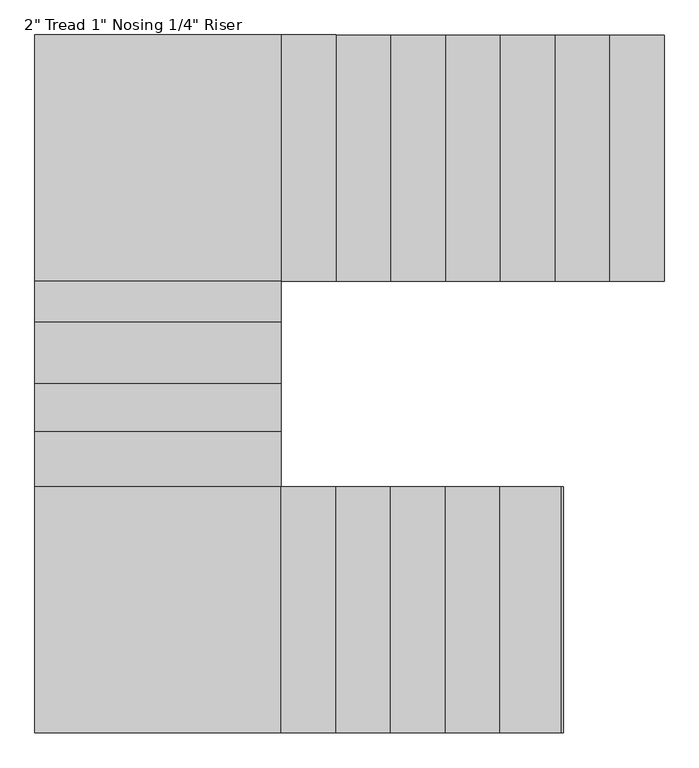
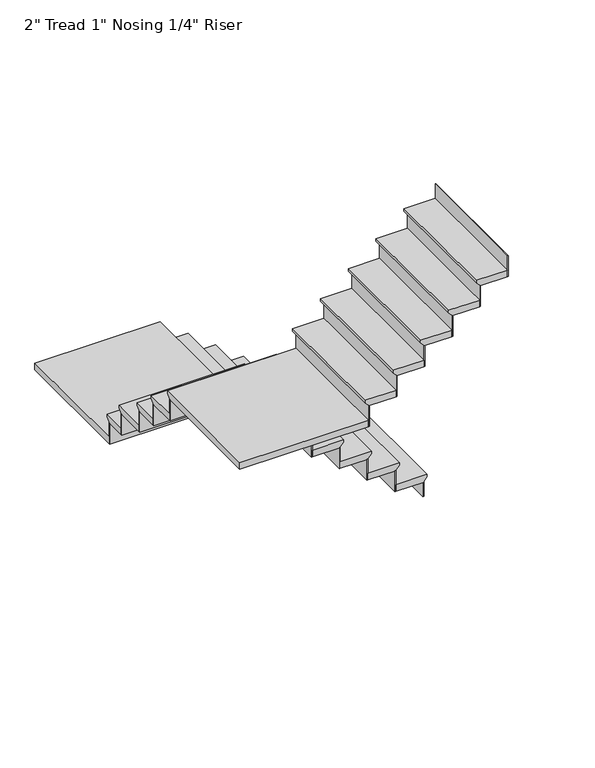
"""IFC4 building model written with IfcOpenShell, lengths in millimetres: stair flight geometry."""

from ifc_helpers import new_model, si_unit, origin, place, context, project, spatial, faceted_brep, source, transform, mapped, element, save


def stair_flight_dc8f8b64(model_context):
    return source(origin(), model_context, "Body", "Brep", [
        faceted_brep([(-3603.1340247, 922.0319954, 16143.3710526), (-3603.1340247, 922.0319954, 16162.4210526), (-3603.1340247, 7.6319954, 16162.4210526), (-3603.1340247, 7.6319954, 16143.3710526), (-3628.5340247, 922.0319954, 16117.9710526), (-3628.5340247, 7.6319954, 16117.9710526), (-3831.7340247, 922.0319954, 16162.4210526), (-3831.7340247, 7.6319954, 16162.4210526), (-3628.5340247, 7.6319954, 16111.6210526), (-3831.7340247, 7.6319954, 16111.6210526), (-3831.7340247, 922.0319954, 16111.6210526), (-3628.5340247, 922.0319954, 16111.6210526)], [[[0, 1, 2, 3]], [[4, 0, 3, 5]], [[2, 1, 6, 7]], [[8, 9, 10, 11]], [[2, 7, 9, 8, 5, 3]], [[8, 11, 4, 5]], [[6, 1, 0, 4, 11, 10]], [[7, 6, 10, 9]]]),
        faceted_brep([(-3628.5340247, 922.0319954, 16111.6210526), (-3628.5340247, 922.0319954, 16002.0), (-3634.8840247, 922.0319954, 16002.0), (-3634.8840247, 922.0319954, 16111.6210526), (-3628.5340247, 7.6319954, 16111.6210526), (-3634.8840247, 7.6319954, 16111.6210526), (-3634.8840247, 7.6319954, 16002.0), (-3628.5340247, 7.6319954, 16002.0)], [[[0, 1, 2, 3]], [[4, 5, 6, 7]], [[1, 0, 4, 7]], [[2, 1, 7, 6]], [[3, 2, 6, 5]], [[0, 3, 5, 4]]]),
        faceted_brep([(-3831.7340247, 922.0319954, 16272.0421053), (-3831.7340247, 922.0319954, 16111.6210526), (-3838.0840247, 922.0319954, 16111.6210526), (-3838.0840247, 922.0319954, 16272.0421053), (-3831.7340247, 7.6319954, 16272.0421053), (-3838.0840247, 7.6319954, 16272.0421053), (-3838.0840247, 7.6319954, 16111.6210526), (-3831.7340247, 7.6319954, 16111.6210526)], [[[0, 1, 2, 3]], [[4, 5, 6, 7]], [[1, 0, 4, 7]], [[2, 1, 7, 6]], [[3, 2, 6, 5]], [[0, 3, 5, 4]]]),
        faceted_brep([(-3806.3340247, 7.6319954, 16322.8421053), (-3806.3340247, 922.0319954, 16322.8421053), (-4034.9340247, 922.0319954, 16322.8421053), (-4034.9340247, 7.6319954, 16322.8421053), (-3831.7340247, 7.6319954, 16272.0421053), (-4034.9340247, 7.6319954, 16272.0421053), (-4034.9340247, 922.0319954, 16272.0421053), (-3831.7340247, 922.0319954, 16272.0421053), (-3831.7340247, 7.6319954, 16278.3921053), (-3806.3340247, 7.6319954, 16303.7921053), (-3831.7340247, 922.0319954, 16278.3921053), (-3806.3340247, 922.0319954, 16303.7921053)], [[[0, 1, 2, 3]], [[4, 5, 6, 7]], [[0, 3, 5, 4, 8, 9]], [[4, 7, 10, 8]], [[2, 1, 11, 10, 7, 6]], [[3, 2, 6, 5]], [[11, 1, 0, 9]], [[10, 11, 9, 8]]]),
        faceted_brep([(-4034.9340247, 922.0319954, 16432.4631579), (-4034.9340247, 922.0319954, 16272.0421053), (-4041.2840247, 922.0319954, 16272.0421053), (-4041.2840247, 922.0319954, 16432.4631579), (-4034.9340247, 7.6319954, 16432.4631579), (-4041.2840247, 7.6319954, 16432.4631579), (-4041.2840247, 7.6319954, 16272.0421053), (-4034.9340247, 7.6319954, 16272.0421053)], [[[0, 1, 2, 3]], [[4, 5, 6, 7]], [[1, 0, 4, 7]], [[2, 1, 7, 6]], [[3, 2, 6, 5]], [[0, 3, 5, 4]]]),
        faceted_brep([(-4009.5340247, 7.6319954, 16483.2631579), (-4009.5340247, 922.0319954, 16483.2631579), (-4238.1340247, 922.0319954, 16483.2631579), (-4238.1340247, 7.6319954, 16483.2631579), (-4034.9340247, 7.6319954, 16432.4631579), (-4238.1340247, 7.6319954, 16432.4631579), (-4238.1340247, 922.0319954, 16432.4631579), (-4034.9340247, 922.0319954, 16432.4631579), (-4034.9340247, 7.6319954, 16438.8131579), (-4009.5340247, 7.6319954, 16464.2131579), (-4034.9340247, 922.0319954, 16438.8131579), (-4009.5340247, 922.0319954, 16464.2131579)], [[[0, 1, 2, 3]], [[4, 5, 6, 7]], [[0, 3, 5, 4, 8, 9]], [[4, 7, 10, 8]], [[2, 1, 11, 10, 7, 6]], [[3, 2, 6, 5]], [[11, 1, 0, 9]], [[10, 11, 9, 8]]]),
        faceted_brep([(-4238.1340247, 922.0319954, 16592.8842105), (-4238.1340247, 922.0319954, 16432.4631579), (-4244.4840247, 922.0319954, 16432.4631579), (-4244.4840247, 922.0319954, 16592.8842105), (-4238.1340247, 7.6319954, 16592.8842105), (-4244.4840247, 7.6319954, 16592.8842105), (-4244.4840247, 7.6319954, 16432.4631579), (-4238.1340247, 7.6319954, 16432.4631579)], [[[0, 1, 2, 3]], [[4, 5, 6, 7]], [[1, 0, 4, 7]], [[2, 1, 7, 6]], [[3, 2, 6, 5]], [[0, 3, 5, 4]]]),
        faceted_brep([(-4212.7340247, 7.6319954, 16643.6842105), (-4212.7340247, 922.0319954, 16643.6842105), (-4441.3340247, 922.0319954, 16643.6842105), (-4441.3340247, 7.6319954, 16643.6842105), (-4238.1340247, 7.6319954, 16592.8842105), (-4441.3340247, 7.6319954, 16592.8842105), (-4441.3340247, 922.0319954, 16592.8842105), (-4238.1340247, 922.0319954, 16592.8842105), (-4238.1340247, 7.6319954, 16599.2342105), (-4212.7340247, 7.6319954, 16624.6342105), (-4238.1340247, 922.0319954, 16599.2342105), (-4212.7340247, 922.0319954, 16624.6342105)], [[[0, 1, 2, 3]], [[4, 5, 6, 7]], [[0, 3, 5, 4, 8, 9]], [[4, 7, 10, 8]], [[2, 1, 11, 10, 7, 6]], [[3, 2, 6, 5]], [[11, 1, 0, 9]], [[10, 11, 9, 8]]]),
        faceted_brep([(-4441.3340247, 922.0319954, 16753.3052632), (-4441.3340247, 922.0319954, 16592.8842105), (-4447.6840247, 922.0319954, 16592.8842105), (-4447.6840247, 922.0319954, 16753.3052632), (-4441.3340247, 7.6319954, 16753.3052632), (-4447.6840247, 7.6319954, 16753.3052632), (-4447.6840247, 7.6319954, 16592.8842105), (-4441.3340247, 7.6319954, 16592.8842105)], [[[0, 1, 2, 3]], [[4, 5, 6, 7]], [[1, 0, 4, 7]], [[2, 1, 7, 6]], [[3, 2, 6, 5]], [[0, 3, 5, 4]]]),
        faceted_brep([(-4415.9340247, 7.6319954, 16804.1052632), (-4415.9340247, 922.0319954, 16804.1052632), (-4644.5340247, 922.0319954, 16804.1052632), (-4644.5340247, 7.6319954, 16804.1052632), (-4441.3340247, 7.6319954, 16753.3052632), (-4644.5340247, 7.6319954, 16753.3052632), (-4644.5340247, 922.0319954, 16753.3052632), (-4441.3340247, 922.0319954, 16753.3052632), (-4441.3340247, 7.6319954, 16759.6552632), (-4415.9340247, 7.6319954, 16785.0552632), (-4441.3340247, 922.0319954, 16759.6552632), (-4415.9340247, 922.0319954, 16785.0552632)], [[[0, 1, 2, 3]], [[4, 5, 6, 7]], [[0, 3, 5, 4, 8, 9]], [[4, 7, 10, 8]], [[2, 1, 11, 10, 7, 6]], [[3, 2, 6, 5]], [[11, 1, 0, 9]], [[10, 11, 9, 8]]]),
        faceted_brep([(-4644.5340247, 922.0319954, 16913.7263158), (-4644.5340247, 922.0319954, 16753.3052632), (-4650.8840247, 922.0319954, 16753.3052632), (-4650.8840247, 922.0319954, 16913.7263158), (-4644.5340247, 7.6319954, 16913.7263158), (-4650.8840247, 7.6319954, 16913.7263158), (-4650.8840247, 7.6319954, 16753.3052632), (-4644.5340247, 7.6319954, 16753.3052632)], [[[0, 1, 2, 3]], [[4, 5, 6, 7]], [[1, 0, 4, 7]], [[2, 1, 7, 6]], [[3, 2, 6, 5]], [[0, 3, 5, 4]]]),
        faceted_brep([(-4619.1340247, 7.6319954, 16964.5263158), (-4619.1340247, 922.0319954, 16964.5263158), (-4847.7340247, 922.0319954, 16964.5263158), (-4847.7340247, 7.6319954, 16964.5263158), (-4644.5340247, 7.6319954, 16913.7263158), (-4847.7340247, 7.6319954, 16913.7263158), (-4847.7340247, 922.0319954, 16913.7263158), (-4644.5340247, 922.0319954, 16913.7263158), (-4644.5340247, 7.6319954, 16920.0763158), (-4619.1340247, 7.6319954, 16945.4763158), (-4644.5340247, 922.0319954, 16920.0763158), (-4619.1340247, 922.0319954, 16945.4763158)], [[[0, 1, 2, 3]], [[4, 5, 6, 7]], [[0, 3, 5, 4, 8, 9]], [[4, 7, 10, 8]], [[2, 1, 11, 10, 7, 6]], [[3, 2, 6, 5]], [[11, 1, 0, 9]], [[10, 11, 9, 8]]]),
        faceted_brep([(-4847.7340247, 922.0319954, 17074.1473684), (-4847.7340247, 922.0319954, 16913.7263158), (-4854.0840247, 922.0319954, 16913.7263158), (-4854.0840247, 922.0319954, 17074.1473684), (-4847.7340247, 7.6319954, 17074.1473684), (-4854.0840247, 7.6319954, 17074.1473684), (-4854.0840247, 7.6319954, 16913.7263158), (-4847.7340247, 7.6319954, 16913.7263158)], [[[0, 1, 2, 3]], [[4, 5, 6, 7]], [[1, 0, 4, 7]], [[2, 1, 7, 6]], [[3, 2, 6, 5]], [[0, 3, 5, 4]]]),
        faceted_brep([(-4822.3340247, 7.6319954, 17124.9473684), (-4822.3340247, 922.0319954, 17124.9473684), (-5050.9340247, 922.0319954, 17124.9473684), (-5050.9340247, 7.6319954, 17124.9473684), (-4847.7340247, 7.6319954, 17074.1473684), (-5050.9340247, 7.6319954, 17074.1473684), (-5050.9340247, 922.0319954, 17074.1473684), (-4847.7340247, 922.0319954, 17074.1473684), (-4847.7340247, 7.6319954, 17080.4973684), (-4822.3340247, 7.6319954, 17105.8973684), (-4847.7340247, 922.0319954, 17080.4973684), (-4822.3340247, 922.0319954, 17105.8973684)], [[[0, 1, 2, 3]], [[4, 5, 6, 7]], [[0, 3, 5, 4, 8, 9]], [[4, 7, 10, 8]], [[2, 1, 11, 10, 7, 6]], [[3, 2, 6, 5]], [[11, 1, 0, 9]], [[10, 11, 9, 8]]]),
        faceted_brep([(-5050.9340247, 922.0319954, 17234.5684211), (-5050.9340247, 922.0319954, 17074.1473684), (-5057.2840247, 922.0319954, 17074.1473684), (-5057.2840247, 922.0319954, 17234.5684211), (-5050.9340247, 7.6319954, 17234.5684211), (-5057.2840247, 7.6319954, 17234.5684211), (-5057.2840247, 7.6319954, 17074.1473684), (-5050.9340247, 7.6319954, 17074.1473684)], [[[0, 1, 2, 3]], [[4, 5, 6, 7]], [[1, 0, 4, 7]], [[2, 1, 7, 6]], [[3, 2, 6, 5]], [[0, 3, 5, 4]]]),
        faceted_brep([(-5939.9340247, 922.0319954, 17285.3684211), (-5939.9340247, -17.7680046, 17285.3684211), (-5025.5340247, -17.7680046, 17285.3684211), (-5025.5340247, 922.0319954, 17285.3684211), (-5025.5340247, 7.6319954, 17234.5684211), (-5025.5340247, -17.7680046, 17234.5684211), (-5939.9340247, -17.7680046, 17234.5684211), (-5939.9340247, 922.0319954, 17234.5684211), (-5050.9340247, 922.0319954, 17234.5684211), (-5050.9340247, 7.6319954, 17234.5684211), (-5025.5340247, 7.6319954, 17266.3184211), (-5025.5340247, 922.0319954, 17266.3184211), (-5050.9340247, 7.6319954, 17240.9184211), (-5050.9340247, 922.0319954, 17240.9184211)], [[[0, 1, 2, 3]], [[4, 5, 6, 7, 8, 9]], [[3, 2, 5, 4, 10, 11]], [[4, 9, 12, 10]], [[9, 8, 13, 12]], [[0, 3, 11, 13, 8, 7]], [[1, 0, 7, 6]], [[2, 1, 6, 5]], [[13, 11, 10, 12]]]),
        faceted_brep([(-5939.9340247, -17.7680046, 17394.9894737), (-5939.9340247, -17.7680046, 17234.5684211), (-5939.9340247, -24.1180046, 17234.5684211), (-5939.9340247, -24.1180046, 17394.9894737), (-5025.5340247, -17.7680046, 17394.9894737), (-5025.5340247, -24.1180046, 17394.9894737), (-5025.5340247, -24.1180046, 17234.5684211), (-5025.5340247, -17.7680046, 17234.5684211)], [[[0, 1, 2, 3]], [[4, 5, 6, 7]], [[1, 0, 4, 7]], [[2, 1, 7, 6]], [[3, 2, 6, 5]], [[0, 3, 5, 4]]]),
        faceted_brep([(-5025.5340247, 7.6319954, 17445.7894737), (-5939.9340247, 7.6319954, 17445.7894737), (-5939.9340247, -170.1680046, 17445.7894737), (-5025.5340247, -170.1680046, 17445.7894737), (-5025.5340247, -17.7680046, 17394.9894737), (-5025.5340247, -170.1680046, 17394.9894737), (-5939.9340247, -170.1680046, 17394.9894737), (-5939.9340247, -17.7680046, 17394.9894737), (-5025.5340247, -17.7680046, 17401.3394737), (-5025.5340247, 7.6319954, 17426.7394737), (-5939.9340247, -17.7680046, 17401.3394737), (-5939.9340247, 7.6319954, 17426.7394737)], [[[0, 1, 2, 3]], [[4, 5, 6, 7]], [[0, 3, 5, 4, 8, 9]], [[4, 7, 10, 8]], [[2, 1, 11, 10, 7, 6]], [[3, 2, 6, 5]], [[11, 1, 0, 9]], [[10, 11, 9, 8]]]),
        faceted_brep([(-5939.9340247, -170.1680046, 17555.4105263), (-5939.9340247, -170.1680046, 17394.9894737), (-5939.9340247, -176.5180046, 17394.9894737), (-5939.9340247, -176.5180046, 17555.4105263), (-5025.5340247, -170.1680046, 17555.4105263), (-5025.5340247, -176.5180046, 17555.4105263), (-5025.5340247, -176.5180046, 17394.9894737), (-5025.5340247, -170.1680046, 17394.9894737)], [[[0, 1, 2, 3]], [[4, 5, 6, 7]], [[1, 0, 4, 7]], [[2, 1, 7, 6]], [[3, 2, 6, 5]], [[0, 3, 5, 4]]]),
        faceted_brep([(-5025.5340247, -144.7680046, 17606.2105263), (-5939.9340247, -144.7680046, 17606.2105263), (-5939.9340247, -398.7680046, 17606.2105263), (-5025.5340247, -398.7680046, 17606.2105263), (-5025.5340247, -170.1680046, 17555.4105263), (-5025.5340247, -398.7680046, 17555.4105263), (-5939.9340247, -398.7680046, 17555.4105263), (-5939.9340247, -170.1680046, 17555.4105263), (-5025.5340247, -170.1680046, 17561.7605263), (-5025.5340247, -144.7680046, 17587.1605263), (-5939.9340247, -170.1680046, 17561.7605263), (-5939.9340247, -144.7680046, 17587.1605263)], [[[0, 1, 2, 3]], [[4, 5, 6, 7]], [[0, 3, 5, 4, 8, 9]], [[4, 7, 10, 8]], [[2, 1, 11, 10, 7, 6]], [[3, 2, 6, 5]], [[11, 1, 0, 9]], [[10, 11, 9, 8]]]),
        faceted_brep([(-5939.9340247, -398.7680046, 17715.8315789), (-5939.9340247, -398.7680046, 17555.4105263), (-5939.9340247, -405.1180046, 17555.4105263), (-5939.9340247, -405.1180046, 17715.8315789), (-5025.5340247, -398.7680046, 17715.8315789), (-5025.5340247, -405.1180046, 17715.8315789), (-5025.5340247, -405.1180046, 17555.4105263), (-5025.5340247, -398.7680046, 17555.4105263)], [[[0, 1, 2, 3]], [[4, 5, 6, 7]], [[1, 0, 4, 7]], [[2, 1, 7, 6]], [[3, 2, 6, 5]], [[0, 3, 5, 4]]]),
        faceted_brep([(-5025.5340247, -373.3680046, 17766.6315789), (-5939.9340247, -373.3680046, 17766.6315789), (-5939.9340247, -576.5680046, 17766.6315789), (-5025.5340247, -576.5680046, 17766.6315789), (-5025.5340247, -398.7680046, 17715.8315789), (-5025.5340247, -576.5680046, 17715.8315789), (-5939.9340247, -576.5680046, 17715.8315789), (-5939.9340247, -398.7680046, 17715.8315789), (-5025.5340247, -398.7680046, 17722.1815789), (-5025.5340247, -373.3680046, 17747.5815789), (-5939.9340247, -398.7680046, 17722.1815789), (-5939.9340247, -373.3680046, 17747.5815789)], [[[0, 1, 2, 3]], [[4, 5, 6, 7]], [[0, 3, 5, 4, 8, 9]], [[4, 7, 10, 8]], [[2, 1, 11, 10, 7, 6]], [[3, 2, 6, 5]], [[11, 1, 0, 9]], [[10, 11, 9, 8]]]),
        faceted_brep([(-5939.9340247, -576.5680046, 17876.2526316), (-5939.9340247, -576.5680046, 17715.8315789), (-5939.9340247, -582.9180046, 17715.8315789), (-5939.9340247, -582.9180046, 17876.2526316), (-5025.5340247, -576.5680046, 17876.2526316), (-5025.5340247, -582.9180046, 17876.2526316), (-5025.5340247, -582.9180046, 17715.8315789), (-5025.5340247, -576.5680046, 17715.8315789)], [[[0, 1, 2, 3]], [[4, 5, 6, 7]], [[1, 0, 4, 7]], [[2, 1, 7, 6]], [[3, 2, 6, 5]], [[0, 3, 5, 4]]]),
        faceted_brep([(-5025.5340247, -551.1680046, 17927.0526316), (-5939.9340247, -551.1680046, 17927.0526316), (-5939.9340247, -779.7680046, 17927.0526316), (-5025.5340247, -779.7680046, 17927.0526316), (-5025.5340247, -576.5680046, 17876.2526316), (-5025.5340247, -779.7680046, 17876.2526316), (-5939.9340247, -779.7680046, 17876.2526316), (-5939.9340247, -576.5680046, 17876.2526316), (-5025.5340247, -576.5680046, 17882.6026316), (-5025.5340247, -551.1680046, 17908.0026316), (-5939.9340247, -576.5680046, 17882.6026316), (-5939.9340247, -551.1680046, 17908.0026316)], [[[0, 1, 2, 3]], [[4, 5, 6, 7]], [[0, 3, 5, 4, 8, 9]], [[4, 7, 10, 8]], [[2, 1, 11, 10, 7, 6]], [[3, 2, 6, 5]], [[11, 1, 0, 9]], [[10, 11, 9, 8]]]),
        faceted_brep([(-5939.9340247, -779.7680046, 18036.6736842), (-5939.9340247, -779.7680046, 17876.2526316), (-5939.9340247, -786.1180046, 17876.2526316), (-5939.9340247, -786.1180046, 18036.6736842), (-5025.5340247, -779.7680046, 18036.6736842), (-5025.5340247, -786.1180046, 18036.6736842), (-5025.5340247, -786.1180046, 17876.2526316), (-5025.5340247, -779.7680046, 17876.2526316)], [[[0, 1, 2, 3]], [[4, 5, 6, 7]], [[1, 0, 4, 7]], [[2, 1, 7, 6]], [[3, 2, 6, 5]], [[0, 3, 5, 4]]]),
        faceted_brep([(-5939.9340247, -1668.7680046, 18087.4736842), (-5000.1340247, -1668.7680046, 18087.4736842), (-5000.1340247, -754.3680046, 18087.4736842), (-5939.9340247, -754.3680046, 18087.4736842), (-5025.5340247, -754.3680046, 18036.6736842), (-5000.1340247, -754.3680046, 18036.6736842), (-5000.1340247, -1668.7680046, 18036.6736842), (-5939.9340247, -1668.7680046, 18036.6736842), (-5939.9340247, -779.7680046, 18036.6736842), (-5025.5340247, -779.7680046, 18036.6736842), (-5025.5340247, -754.3680046, 18068.4236842), (-5939.9340247, -754.3680046, 18068.4236842), (-5025.5340247, -779.7680046, 18043.0236842), (-5939.9340247, -779.7680046, 18043.0236842)], [[[0, 1, 2, 3]], [[4, 5, 6, 7, 8, 9]], [[3, 2, 5, 4, 10, 11]], [[4, 9, 12, 10]], [[9, 8, 13, 12]], [[0, 3, 11, 13, 8, 7]], [[1, 0, 7, 6]], [[2, 1, 6, 5]], [[13, 11, 10, 12]]]),
        faceted_brep([(-5000.1340247, -1668.7680046, 18197.0947368), (-5000.1340247, -1668.7680046, 18036.6736842), (-4993.7840247, -1668.7680046, 18036.6736842), (-4993.7840247, -1668.7680046, 18197.0947368), (-5000.1340247, -754.3680046, 18197.0947368), (-4993.7840247, -754.3680046, 18197.0947368), (-4993.7840247, -754.3680046, 18036.6736842), (-5000.1340247, -754.3680046, 18036.6736842)], [[[0, 1, 2, 3]], [[4, 5, 6, 7]], [[1, 0, 4, 7]], [[2, 1, 7, 6]], [[3, 2, 6, 5]], [[0, 3, 5, 4]]]),
        faceted_brep([(-5025.5340247, -754.3680046, 18247.8947368), (-5025.5340247, -1668.7680046, 18247.8947368), (-4796.9340247, -1668.7680046, 18247.8947368), (-4796.9340247, -754.3680046, 18247.8947368), (-5000.1340247, -754.3680046, 18197.0947368), (-4796.9340247, -754.3680046, 18197.0947368), (-4796.9340247, -1668.7680046, 18197.0947368), (-5000.1340247, -1668.7680046, 18197.0947368), (-5000.1340247, -754.3680046, 18203.4447368), (-5025.5340247, -754.3680046, 18228.8447368), (-5000.1340247, -1668.7680046, 18203.4447368), (-5025.5340247, -1668.7680046, 18228.8447368)], [[[0, 1, 2, 3]], [[4, 5, 6, 7]], [[0, 3, 5, 4, 8, 9]], [[4, 7, 10, 8]], [[2, 1, 11, 10, 7, 6]], [[3, 2, 6, 5]], [[11, 1, 0, 9]], [[10, 11, 9, 8]]]),
        faceted_brep([(-4796.9340247, -1668.7680046, 18357.5157895), (-4796.9340247, -1668.7680046, 18197.0947368), (-4790.5840247, -1668.7680046, 18197.0947368), (-4790.5840247, -1668.7680046, 18357.5157895), (-4796.9340247, -754.3680046, 18357.5157895), (-4790.5840247, -754.3680046, 18357.5157895), (-4790.5840247, -754.3680046, 18197.0947368), (-4796.9340247, -754.3680046, 18197.0947368)], [[[0, 1, 2, 3]], [[4, 5, 6, 7]], [[1, 0, 4, 7]], [[2, 1, 7, 6]], [[3, 2, 6, 5]], [[0, 3, 5, 4]]]),
        faceted_brep([(-4822.3340247, -754.3680046, 18408.3157895), (-4822.3340247, -1668.7680046, 18408.3157895), (-4593.7340247, -1668.7680046, 18408.3157895), (-4593.7340247, -754.3680046, 18408.3157895), (-4796.9340247, -754.3680046, 18357.5157895), (-4593.7340247, -754.3680046, 18357.5157895), (-4593.7340247, -1668.7680046, 18357.5157895), (-4796.9340247, -1668.7680046, 18357.5157895), (-4796.9340247, -754.3680046, 18363.8657895), (-4822.3340247, -754.3680046, 18389.2657895), (-4796.9340247, -1668.7680046, 18363.8657895), (-4822.3340247, -1668.7680046, 18389.2657895)], [[[0, 1, 2, 3]], [[4, 5, 6, 7]], [[0, 3, 5, 4, 8, 9]], [[4, 7, 10, 8]], [[2, 1, 11, 10, 7, 6]], [[3, 2, 6, 5]], [[11, 1, 0, 9]], [[10, 11, 9, 8]]]),
        faceted_brep([(-4593.7340247, -1668.7680046, 18517.9368421), (-4593.7340247, -1668.7680046, 18357.5157895), (-4587.3840247, -1668.7680046, 18357.5157895), (-4587.3840247, -1668.7680046, 18517.9368421), (-4593.7340247, -754.3680046, 18517.9368421), (-4587.3840247, -754.3680046, 18517.9368421), (-4587.3840247, -754.3680046, 18357.5157895), (-4593.7340247, -754.3680046, 18357.5157895)], [[[0, 1, 2, 3]], [[4, 5, 6, 7]], [[1, 0, 4, 7]], [[2, 1, 7, 6]], [[3, 2, 6, 5]], [[0, 3, 5, 4]]]),
        faceted_brep([(-4619.1340247, -754.3680046, 18568.7368421), (-4619.1340247, -1668.7680046, 18568.7368421), (-4390.5340247, -1668.7680046, 18568.7368421), (-4390.5340247, -754.3680046, 18568.7368421), (-4593.7340247, -754.3680046, 18517.9368421), (-4390.5340247, -754.3680046, 18517.9368421), (-4390.5340247, -1668.7680046, 18517.9368421), (-4593.7340247, -1668.7680046, 18517.9368421), (-4593.7340247, -754.3680046, 18524.2868421), (-4619.1340247, -754.3680046, 18549.6868421), (-4593.7340247, -1668.7680046, 18524.2868421), (-4619.1340247, -1668.7680046, 18549.6868421)], [[[0, 1, 2, 3]], [[4, 5, 6, 7]], [[0, 3, 5, 4, 8, 9]], [[4, 7, 10, 8]], [[2, 1, 11, 10, 7, 6]], [[3, 2, 6, 5]], [[11, 1, 0, 9]], [[10, 11, 9, 8]]]),
        faceted_brep([(-4390.5340247, -1668.7680046, 18678.3578947), (-4390.5340247, -1668.7680046, 18517.9368421), (-4384.1840247, -1668.7680046, 18517.9368421), (-4384.1840247, -1668.7680046, 18678.3578947), (-4390.5340247, -754.3680046, 18678.3578947), (-4384.1840247, -754.3680046, 18678.3578947), (-4384.1840247, -754.3680046, 18517.9368421), (-4390.5340247, -754.3680046, 18517.9368421)], [[[0, 1, 2, 3]], [[4, 5, 6, 7]], [[1, 0, 4, 7]], [[2, 1, 7, 6]], [[3, 2, 6, 5]], [[0, 3, 5, 4]]]),
        faceted_brep([(-4415.9340247, -754.3680046, 18729.1578947), (-4415.9340247, -1668.7680046, 18729.1578947), (-4187.3340247, -1668.7680046, 18729.1578947), (-4187.3340247, -754.3680046, 18729.1578947), (-4390.5340247, -754.3680046, 18678.3578947), (-4187.3340247, -754.3680046, 18678.3578947), (-4187.3340247, -1668.7680046, 18678.3578947), (-4390.5340247, -1668.7680046, 18678.3578947), (-4390.5340247, -754.3680046, 18684.7078947), (-4415.9340247, -754.3680046, 18710.1078947), (-4390.5340247, -1668.7680046, 18684.7078947), (-4415.9340247, -1668.7680046, 18710.1078947)], [[[0, 1, 2, 3]], [[4, 5, 6, 7]], [[0, 3, 5, 4, 8, 9]], [[4, 7, 10, 8]], [[2, 1, 11, 10, 7, 6]], [[3, 2, 6, 5]], [[11, 1, 0, 9]], [[10, 11, 9, 8]]]),
        faceted_brep([(-4187.3340247, -1668.7680046, 18838.7789474), (-4187.3340247, -1668.7680046, 18678.3578947), (-4180.9840247, -1668.7680046, 18678.3578947), (-4180.9840247, -1668.7680046, 18838.7789474), (-4187.3340247, -754.3680046, 18838.7789474), (-4180.9840247, -754.3680046, 18838.7789474), (-4180.9840247, -754.3680046, 18678.3578947), (-4187.3340247, -754.3680046, 18678.3578947)], [[[0, 1, 2, 3]], [[4, 5, 6, 7]], [[1, 0, 4, 7]], [[2, 1, 7, 6]], [[3, 2, 6, 5]], [[0, 3, 5, 4]]]),
        faceted_brep([(-3984.1340247, -1668.7680046, 18999.2), (-3984.1340247, -1668.7680046, 18838.7789474), (-3977.7840247, -1668.7680046, 18838.7789474), (-3977.7840247, -1668.7680046, 18999.2), (-3984.1340247, -754.3680046, 18999.2), (-3977.7840247, -754.3680046, 18999.2), (-3977.7840247, -754.3680046, 18838.7789474), (-3984.1340247, -754.3680046, 18838.7789474)], [[[0, 1, 2, 3]], [[4, 5, 6, 7]], [[1, 0, 4, 7]], [[2, 1, 7, 6]], [[3, 2, 6, 5]], [[0, 3, 5, 4]]]),
        faceted_brep([(-4212.7340247, -754.3680046, 18889.5789474), (-4212.7340247, -1668.7680046, 18889.5789474), (-3984.1340247, -1668.7680046, 18889.5789474), (-3984.1340247, -754.3680046, 18889.5789474), (-4187.3340247, -754.3680046, 18838.7789474), (-3984.1340247, -754.3680046, 18838.7789474), (-3984.1340247, -1668.7680046, 18838.7789474), (-4187.3340247, -1668.7680046, 18838.7789474), (-4187.3340247, -754.3680046, 18845.1289474), (-4212.7340247, -754.3680046, 18870.5289474), (-4187.3340247, -1668.7680046, 18845.1289474), (-4212.7340247, -1668.7680046, 18870.5289474)], [[[0, 1, 2, 3]], [[4, 5, 6, 7]], [[0, 3, 5, 4, 8, 9]], [[4, 7, 10, 8]], [[2, 1, 11, 10, 7, 6]], [[3, 2, 6, 5]], [[11, 1, 0, 9]], [[10, 11, 9, 8]]]),
    ])


if __name__ == "__main__":
    model = new_model("IFC4")
    model_context = context("Model", 3, world=origin())
    ifc_project = project(units=[si_unit("LENGTHUNIT", "METRE", prefix="MILLI")], contexts=[model_context])
    site = spatial("IfcSite", under=ifc_project)
    building = spatial("IfcBuilding", under=site)
    placement = place(None, origin())
    stair_flight_shape = stair_flight_dc8f8b64(model_context)
    element("IfcStairFlight", 1, ObjectType="2\" Tread 1\" Nosing 1/4\" Riser", at=placement, inside=building, context=model_context, shape_type="MappedRepresentation", body=[
        mapped(stair_flight_shape, transform((0.0, 0.0, 0.0), x_axis=(1.0, 0.0, 0.0), y_axis=(0.0, 1.0, 0.0), z_axis=(0.0, 0.0, 1.0))),
    ])
    save(model, "model.ifc")
